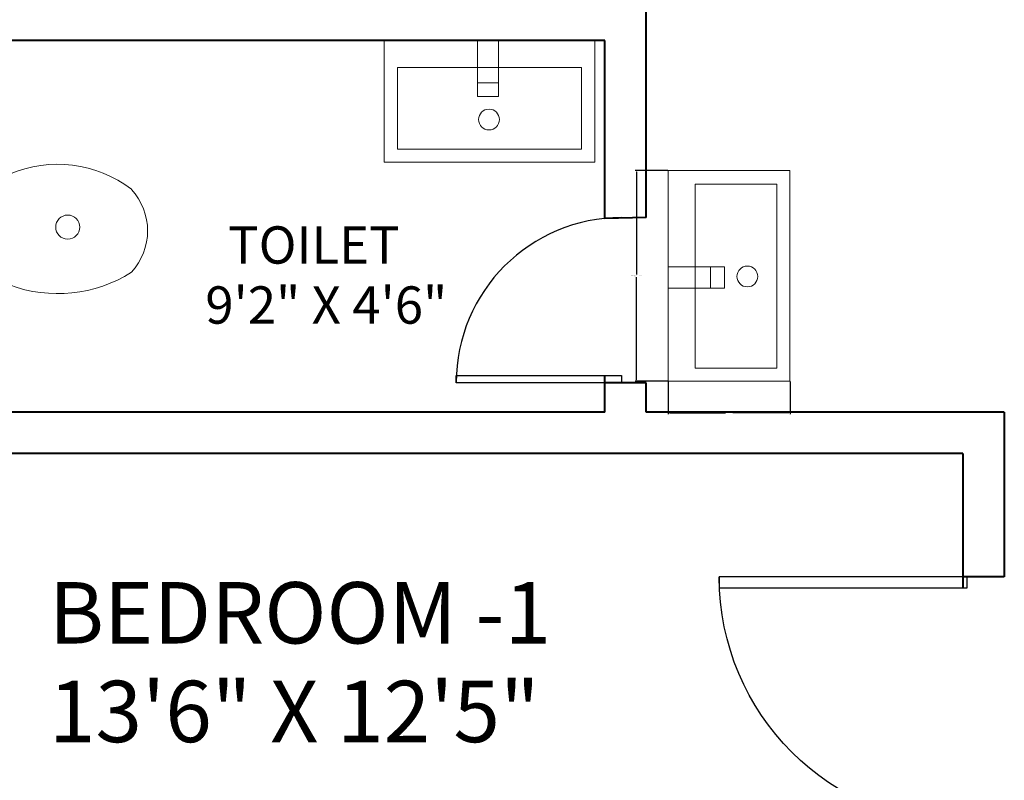
# Model space of a CAD drawing. Units: inches. Extents: x -46 to 1145, y -527 to 760.
# Tile 33 of 57: x 47 to 190, y 332 to 443. Entities that reach past the tile are written whole.
import ezdxf

# ---------------------------------------------------------------- set-up
doc = ezdxf.new("R2010")
doc.units = ezdxf.units.IN
doc.header["$MEASUREMENT"] = 0
for name, color, linetype, lineweight in [('A-ANNO-DIMS', 2, 'Continuous', 18), ('A-AREA-IDEN', 1, 'Continuous', 18), ('A-FLOR-FIXT', 9, 'Continuous', 18), ('DOORS', 3, 'Continuous', 25), ('WALLS', 4, 'Continuous', 40)]:
    doc.layers.add(name, color=color, linetype=linetype, lineweight=lineweight)
doc.styles.get("Standard").update_dxf_attribs({"font": 'arial.ttf'})
doc.dimstyles.get("Standard").update_dxf_attribs({"dimtxt": 0.18, "dimasz": 0.18, "dimexe": 0.18, "dimexo": 0.0625, "dimgap": 0.09, "dimtad": 0, "dimtih": 1, "dimtoh": 1, "dimdec": 0, "dimzin": 0, "dimdsep": 46, "dimlunit": 3, "dimtxsty": 'Standard', "dimcen": 0.09, "dimadec": 0, "dimazin": 0, "dimtfac": 1, "dimtdec": 0, "dimtofl": 0, "dimtmove": 0, "dimatfit": 3, "dimfxl": 1, "dimtolj": 1, "dimtzin": 0, "dimarcsym": 0})

# ---------------------------------------------------------------- blocks, each defined once
blk = doc.blocks.new('*U2')
for p, q in [((0, 0), (0, -6)), ((40, 0), (40, -6))]:
    blk.add_line(p, q)
blk.add_lwpolyline([(0, 0), (0, 40), (1.75, 40), (1.75, 0)], close=True)
blk.add_arc((0, 0), 40, 0, 90)
blk = doc.blocks.new('LAVATORY-RECT')
blk.add_line((14.01, 6.17), (17.08, 6.17))
for points in [[(30.61, 0), (0, 0), (0, 17.7), (30.61, 17.7)], [(28.7, 3.94), (1.97, 3.94), (1.97, 15.81), (28.7, 15.81)], [(17.08, 0), (14.01, 0), (14.01, 8.17), (17.08, 8.17)]]:
    blk.add_lwpolyline(points, close=True)
blk.add_circle((15.39, 11.51), 1.51)
blk = doc.blocks.new('WATER-CLOSET')
for p, q in [((0, 0), (0, 26.01)), ((0, 26.01), (6.13, 26.01)), ((5.22, 21.04), (5.22, 26.01)), ((5.22, 26.01), (5.22, 0)), ((0, 0), (6.13, 0))]:
    blk.add_line(p, q)
blk.add_lwpolyline([(1.51, 11.4), (1.51, 16.16), (3.34, 16.16), (3.34, 11.4)], close=True)
blk.add_circle((19.79, 13.37), 1.75)
for centre, radius, start, end in [((14.15, 29.2), 8.64, 201.6782, 251.0259), ((18.35, 4.96), 17.54, 52.4616, 113.5359), ((22.52, 12.84), 8.87, 317.2682, 42.7318), ((18.33, 23.71), 20, 249.5645, 302.3709), ((15.4, -4.5), 10.31, 113.1704, 154.0947)]:
    blk.add_arc(centre, radius, start, end)
blk = doc.blocks.new('*D658')
at = {"layer": 'A-ANNO-DIMS', "color": 0, "lineweight": -2, "transparency": 16777216}
for p, q in [((140.67, 420.6), (135.96, 420.6)), ((136.14, 420.42), (136.14, 405.48)), ((136.14, 390.18), (136.14, 405.12)), ((140.67, 390), (135.96, 390))]:
    blk.add_line(p, q, dxfattribs=at)
at = {"layer": 'A-ANNO-DIMS', "color": 0, "transparency": 16777216}
for points in [[(136.11, 420.42), (136.17, 420.42), (136.14, 420.6)], [(136.11, 390.18), (136.17, 390.18), (136.14, 390)]]:
    blk.add_solid(points, dxfattribs=at)
at = {"layer": 'Defpoints', "color": 0, "transparency": 16777216}
for p in [(140.74, 420.6), (136.14, 390), (140.74, 390)]:
    blk.add_point(p, dxfattribs=at)
at = {"layer": 'A-ANNO-DIMS', "color": 0, "transparency": 16777216, "insert": (136.14, 405.3), "char_height": 0.18, "attachment_point": 5}
blk.add_mtext('\\A1;BASIN 31 TYP.', dxfattribs=at)
blk = doc.blocks.new('*D659')
at = {"layer": 'A-ANNO-DIMS', "color": 0, "lineweight": -2, "transparency": 16777216}
for p, q in [((140.74, 389.94), (140.74, 385.23)), ((158.44, 389.94), (158.44, 385.23)), ((140.92, 385.41), (149.07, 385.41)), ((158.26, 385.41), (150.11, 385.41))]:
    blk.add_line(p, q, dxfattribs=at)
at = {"layer": 'A-ANNO-DIMS', "color": 0, "transparency": 16777216}
for points in [[(140.92, 385.44), (140.92, 385.38), (140.74, 385.41)], [(158.26, 385.44), (158.26, 385.38), (158.44, 385.41)]]:
    blk.add_solid(points, dxfattribs=at)
at = {"layer": 'Defpoints', "color": 0, "transparency": 16777216}
for p in [(140.74, 390), (158.44, 390), (158.44, 385.41)]:
    blk.add_point(p, dxfattribs=at)
at = {"layer": 'A-ANNO-DIMS', "color": 0, "transparency": 16777216, "insert": (149.59, 385.41), "char_height": 0.18, "attachment_point": 5}
blk.add_mtext('\\A1;18 TYP.', dxfattribs=at)
blk = doc.blocks.new('*D685')
at = {"layer": 'A-ANNO-DIMS', "color": 0, "lineweight": -2, "transparency": 16777216}
for p, q in [((183.5, 700.89), (-46.22, 700.89)), ((-46.04, 700.71), (-46.04, 116.39)), ((-46.04, -468.3), (-46.04, 116.02)), ((12.5, -468.48), (-46.22, -468.48))]:
    blk.add_line(p, q, dxfattribs=at)
at = {"layer": 'A-ANNO-DIMS', "color": 0, "transparency": 16777216}
for points in [[(-46.07, 700.71), (-46.01, 700.71), (-46.04, 700.89)], [(-46.07, -468.3), (-46.01, -468.3), (-46.04, -468.48)]]:
    blk.add_solid(points, dxfattribs=at)
at = {"layer": 'Defpoints', "color": 0, "transparency": 16777216}
for p in [(-46.04, 700.89), (183.56, 700.89), (12.56, -468.48)]:
    blk.add_point(p, dxfattribs=at)
at = {"layer": 'A-ANNO-DIMS', "color": 0, "transparency": 16777216, "insert": (-46.04, 116.2), "char_height": 0.18, "attachment_point": 5}
blk.add_mtext('\\A1;1169.4', dxfattribs=at)

msp = doc.modelspace()

# ---------------------------------------------------------------- linework, layer by layer
at = {"layer": 'WALLS'}
for p, q in [((137.5637, 439.5176), (137.5637, 500.5176)), ((131.5637, 439.5176), (21.5637, 439.5176)), ((131.5637, 413.6562), (131.5637, 439.5176)), ((137.5637, 413.7765), (137.5637, 439.5176)), ((137.5637, 413.7765), (131.5637, 413.6562)), ((131.5637, 385.5176), (131.5637, 390.8265)), ((137.5637, 389.7765), (131.5637, 389.7765)), ((137.5637, 385.5176), (137.5637, 389.7765)), ((131.5637, 385.5176), (21.5637, 385.5176)), ((189.5637, 385.5176), (137.5637, 385.5176)), ((189.5637, 385.5176), (189.5637, 361.5613)), ((183.5637, 379.5176), (21.5637, 379.5176)), ((183.5637, 379.5176), (183.5637, 359.9863)), ((189.5637, 361.5613), (183.5637, 361.5613))]:
    msp.add_line(p, q, dxfattribs=at)

# ---------------------------------------------------------------- block references
at = {"layer": 'A-FLOR-FIXT'}
for p, rotation in [((130.111, 439.5176), 180), ((140.7357, 420.605), 269.9999999999997)]:
    msp.add_blockref('LAVATORY-RECT', p, dxfattribs=dict(at, rotation=rotation))
msp.add_blockref('WATER-CLOSET', (33.743, 399.011), dxfattribs=at)
at = {"layer": 'DOORS', "rotation": 90}
for p, xscale, yscale, zscale in [((133.9637, 389.7765), 0.6, 0.6, 0.6), ((184.1637, 361.5613), -0.9, 0.9, 0.9)]:
    msp.add_blockref('*U2', p, dxfattribs=dict(at, xscale=xscale, yscale=yscale, zscale=zscale))

# ---------------------------------------------------------------- texts
at = {"layer": 'A-AREA-IDEN'}
for s, height, p in [('   TOILET', 5.42821, (71.8549, 407.0717)), (' 9\'2" X 4\'6"', 5.428214, (71.8549, 398.3518)), ('BEDROOM -1 ', 8.923264, (50.8065, 351.892)), ('13\'6" X 12\'5"', 8.923264, (50.8065, 337.5576))]:
    msp.add_text(s, height=height, dxfattribs=at).set_placement(p)

# ---------------------------------------------------------------- dimensions: what is measured, and where the dimension line sits
at = {"layer": 'A-ANNO-DIMS'}
dim = msp.add_linear_dim(base=(-46.0363, 700.8886), p1=(12.5637, -468.4824), p2=(183.5637, 700.8886), angle=90, dimstyle='Standard', override={"dimdec": 1, "dimlfac": 1, "dimrnd": 0, "dimzin": 0, "dimdsep": 46, "dimlunit": 2}, dxfattribs=at)
dim.commit()
dim.dimension.update_dxf_attribs({"geometry": '*D685', "text_midpoint": (-46.0363, 116.2031)})
dim = msp.add_linear_dim(base=(136.1448, 389.9989), p1=(140.7357, 420.6046), p2=(140.7357, 389.9989), angle=270, text='BASIN <> TYP.', dimstyle='Standard', override={"dimdec": 0, "dimlfac": 1, "dimrnd": 0, "dimzin": 0, "dimdsep": 46, "dimlunit": 2}, dxfattribs=at)
dim.commit()
dim.dimension.update_dxf_attribs({"geometry": '*D658', "text_midpoint": (136.1448, 405.3018)})
dim = msp.add_linear_dim(base=(158.4383, 385.408), p1=(140.7357, 389.9989), p2=(158.4383, 389.9989), text='<> TYP.', dimstyle='Standard', override={"dimdec": 0, "dimlfac": 1, "dimrnd": 0, "dimzin": 0, "dimdsep": 46, "dimlunit": 2}, dxfattribs=at)
dim.commit()
dim.dimension.update_dxf_attribs({"geometry": '*D659', "text_midpoint": (149.587, 385.408)})

doc.saveas('drawing.dxf')
